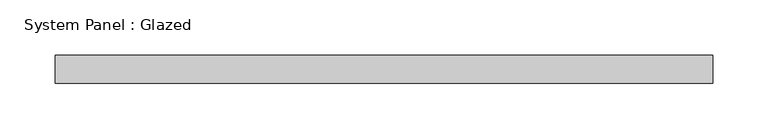
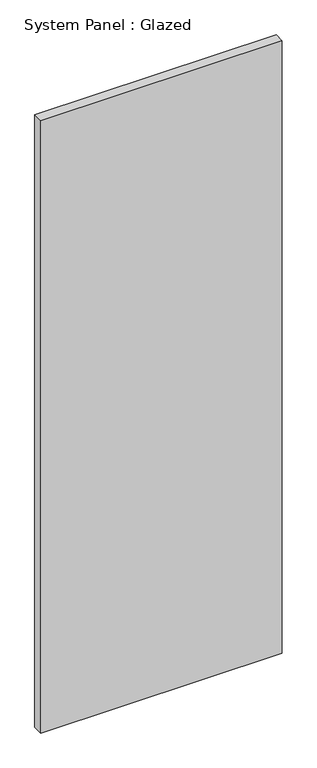
"""IFC4 building model written with IfcOpenShell, lengths in millimetres: plate geometry, System Panel : Glazed."""

from ifc_helpers import new_model, si_unit, origin, origin_with_axes, place, context, project, spatial, polyline, outline, extrude, source, transform, mapped, element, save


def system_panel_glazed_7d7b3bbd(model_context):
    return source(origin(), model_context, "Body", "SweptSolid", [
        extrude(outline(polyline([(298.45, 19.05), (-298.45, 19.05), (-298.45, 44.45), (298.45, 44.45), (298.45, 19.05)])), origin_with_axes(), (0.0, 0.0, 1.0), 1598.9311114),
    ])


if __name__ == "__main__":
    model = new_model("IFC4")
    model_context = context("Model", 3, world=origin())
    ifc_project = project(units=[si_unit("LENGTHUNIT", "METRE", prefix="MILLI")], contexts=[model_context])
    site = spatial("IfcSite", under=ifc_project)
    building = spatial("IfcBuilding", under=site)
    placement = place(None, origin())
    system_panel_glazed_shape = system_panel_glazed_7d7b3bbd(model_context)
    element("IfcPlate", 1, ObjectType="System Panel : Glazed", at=placement, inside=building, context=model_context, shape_type="MappedRepresentation", body=[
        mapped(system_panel_glazed_shape, transform((0.0, 0.0, 0.0), x_axis=(1.0, 0.0, 0.0), y_axis=(0.0, 1.0, 0.0), z_axis=(0.0, 0.0, 1.0))),
    ])
    save(model, "model.ifc")

# Revit data of these elements
# Type "System Panel : Glazed"
#   Construction Type Id = "GSP4R"
#   Analytic Construction = "1/8 in Pilkington single glazing"
#   Visual Light Transmittance = 0.9
#   Solar Heat Gain Coefficient = 0.86
#   Heat Transfer Coefficient (U) = 1.18115 BTU/(h·ft²·°F)
#   Define Thermal Properties by = 1
# Element 1 (IfcPlate, "System Panel : Glazed")
#   Materials on its faces: "Glass"
# Materials
#   "Glass": class "Glass", colour RGB 0 128 192, transparency 0.75, Description = "Soda Lime Glass", Cost = 0
